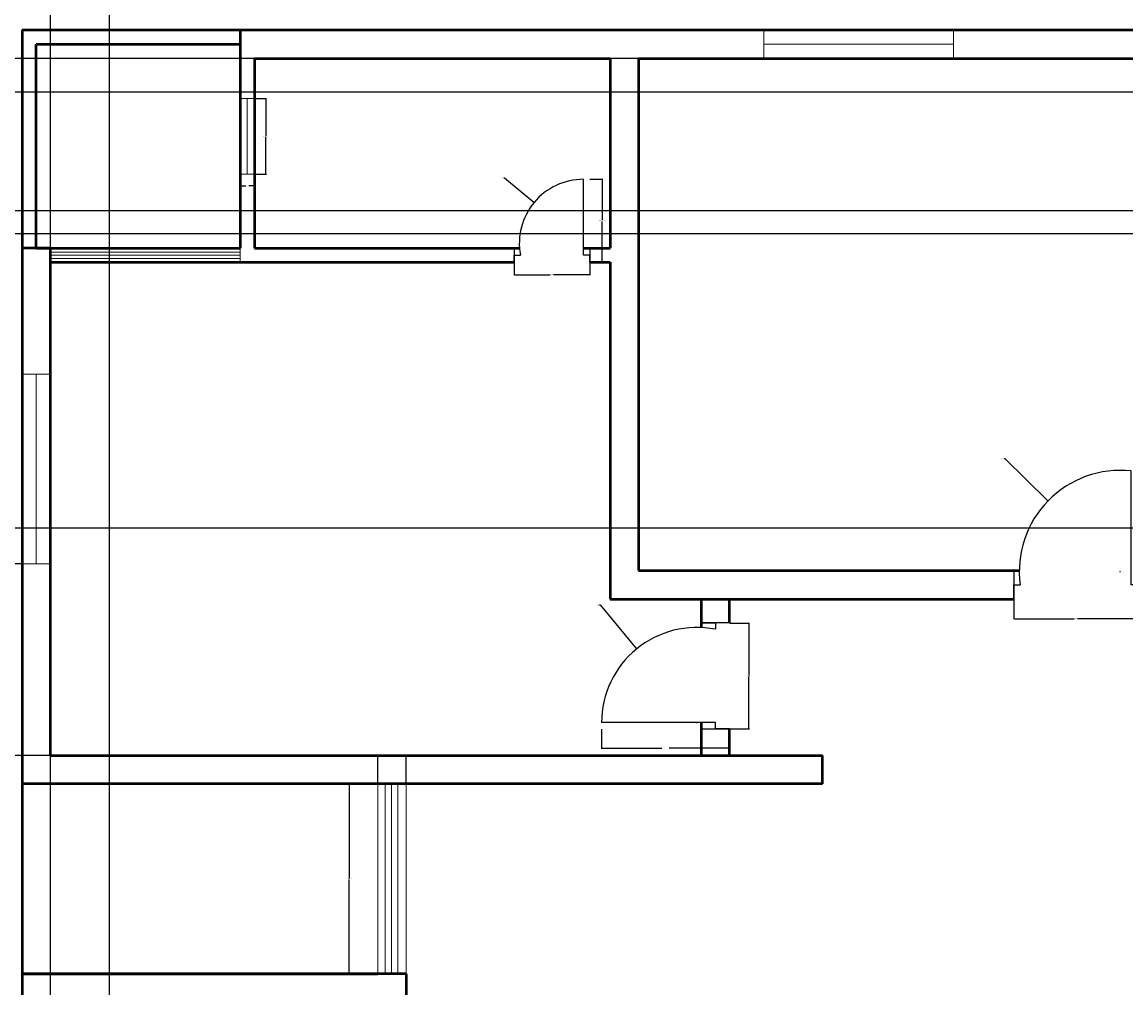
# Model space of a CAD drawing. Units: inches. Extents: x 2215 to 3724, y 1009 to 2124.
# Tile 9 of 11: x 2963 to 3312, y 1444 to 1750. Entities that reach past the tile are written whole.
import ezdxf

# ---------------------------------------------------------------- set-up
doc = ezdxf.new("R2010")
doc.units = ezdxf.units.IN
for name, color, linetype, lineweight in [('A-ANNO-DIMS', 2, 'Continuous', 18), ('A-ANNO-SYMB', 7, 'Continuous', 25), ('A-DOOR', 3, 'Continuous', 25), ('A-GLAZ', 4, 'Continuous', 18), ('A-WALL', 7, 'Continuous', 50)]:
    doc.layers.add(name, color=color, linetype=linetype, lineweight=lineweight)
doc.styles.get("Standard").update_dxf_attribs({"font": 'arial.ttf'})
doc.dimstyles.get("Standard").update_dxf_attribs({"dimtxt": 0.18, "dimasz": 0.18, "dimexe": 0.18, "dimexo": 0.0625, "dimgap": 0.09, "dimtad": 0, "dimtih": 1, "dimtoh": 1, "dimdec": 4, "dimzin": 0, "dimdsep": 46, "dimtxsty": 'Standard', "dimcen": 0.09, "dimadec": 0, "dimazin": 0, "dimtfac": 1, "dimtdec": 4, "dimtofl": 0, "dimtmove": 0, "dimatfit": 3, "dimfxl": 1, "dimtolj": 1, "dimtzin": 0, "dimarcsym": 0})

# ---------------------------------------------------------------- blocks, each defined once
blk = doc.blocks.new('DOOR-BEDROOM-N')
for p, q in [((37.14, 4.5), (37.14, 40.5)), ((0, 9), (0, 0)), ((39.14, 9), (39.14, 0)), ((0, 0), (0, 4.5)), ((0, 4.5), (2, 4.5)), ((39.14, 4.5), (37.14, 4.5)), ((39.14, 0), (39.14, 4.5))]:
    blk.add_line(p, q)
blk.add_arc((33.66, 8.74), 31.95, 83.7441, 187.635)
blk = doc.blocks.new('DOOR-BATH-NW')
for p, q in [((21.95, 2.25), (21.95, 26.25)), ((0, 4.5), (0, 0)), ((23.95, 4.5), (23.95, 0)), ((0, 0), (0, 2.25)), ((0, 2.25), (2, 2.25)), ((23.95, 2.25), (21.95, 2.25)), ((23.95, 0), (23.95, 2.25))]:
    blk.add_line(p, q)
blk.add_arc((21.95, 5.96), 20.29, 90, 190.5328)
blk = doc.blocks.new('DOOR-BEDROOM-W')
for p, q in [((40.5, 33.52), (31.5, 33.52)), ((31.5, 33.52), (36, 33.52)), ((36, 33.52), (36, 31.52)), ((36, 2), (0, 2)), ((31.5, 0), (40.5, 0)), ((36, 0), (36, 2)), ((40.5, 0), (36, 0))]:
    blk.add_line(p, q)
blk.add_arc((30.1, 2), 30.1, 78.701, 180)
blk = doc.blocks.new('WIN-60-JAMB-A')
for p, q in [((0, 9), (0, 0)), ((60, 4.5), (60, 9)), ((60, 9), (60, 0)), ((0, 0), (0, 4.5)), ((0, 4.5), (60, 4.5))]:
    blk.add_line(p, q)
blk = doc.blocks.new('SCREEN-LAUNDRY')
for p, q in [((0, 0), (0, 60)), ((0, 60), (9, 60)), ((4.37, 60), (2.37, 60)), ((2.37, 60), (2.37, 0)), ((4.37, 0), (4.37, 60)), ((6.37, 0), (6.37, 60)), ((9, 60), (9, 0)), ((2.37, 0), (4.37, 0)), ((9, 0), (4.37, 0)), ((4.37, 0), (6.37, 0))]:
    blk.add_line(p, q)
blk = doc.blocks.new('VENT-24-NW')
for p, q in [((0, 24), (0, 24)), ((0, 24), (4.5, 24)), ((4.5, 24), (0, 24)), ((0, 24), (2.25, 24)), ((2.25, 24), (2.25, 0)), ((2.25, 0), (0, 0)), ((0, 0), (0, 0)), ((0, 0), (4.5, 0))]:
    blk.add_line(p, q)
blk = doc.blocks.new('WIN-OTS-W')
for p, q in [((60, 4.5), (60, 0)), ((0, 2.25), (0, 3.25)), ((0, 3.25), (60, 3.25)), ((60, 2.25), (0, 2.25)), ((60, 1.25), (0, 1.25)), ((60, 3.25), (60, 2.25)), ((60, 0), (60, 2.25)), ((60, 2.25), (60, 1.25))]:
    blk.add_line(p, q)
blk = doc.blocks.new('*D39')
at = {"layer": 'A-ANNO-DIMS', "color": 0, "lineweight": -2, "transparency": 16777216}
for p, q in [((3075.18, 1509), (3066.06, 1509)), ((3066.24, 1508.82), (3066.24, 1479.18)), ((3066.24, 1449.18), (3066.24, 1478.81)), ((3075.18, 1449), (3066.06, 1449))]:
    blk.add_line(p, q, dxfattribs=at)
at = {"layer": 'A-ANNO-DIMS', "color": 0, "transparency": 16777216}
for points in [[(3066.21, 1508.82), (3066.27, 1508.82), (3066.24, 1509)], [(3066.21, 1449.18), (3066.27, 1449.18), (3066.24, 1449)]]:
    blk.add_solid(points, dxfattribs=at)
at = {"layer": 'Defpoints', "color": 0, "transparency": 16777216}
for p in [(3066.24, 1509), (3075.24, 1509), (3075.24, 1449)]:
    blk.add_point(p, dxfattribs=at)
at = {"layer": 'A-ANNO-DIMS', "color": 0, "transparency": 16777216, "insert": (3066.24, 1479), "char_height": 0.18, "attachment_point": 5}
blk.add_mtext('\\A1;SCREEN 60 TYP.', dxfattribs=at)
blk = doc.blocks.new('*D40')
at = {"layer": 'A-ANNO-DIMS', "color": 0, "lineweight": -2, "transparency": 16777216}
for p, q in [((3075.24, 1509.06), (3075.24, 1518.18)), ((3075.42, 1518), (3079.29, 1518)), ((3084.06, 1518), (3080.2, 1518)), ((3084.24, 1509.06), (3084.24, 1518.18))]:
    blk.add_line(p, q, dxfattribs=at)
at = {"layer": 'A-ANNO-DIMS', "color": 0, "transparency": 16777216}
for points in [[(3075.42, 1518.03), (3075.42, 1517.97), (3075.24, 1518)], [(3084.06, 1518.03), (3084.06, 1517.97), (3084.24, 1518)]]:
    blk.add_solid(points, dxfattribs=at)
at = {"layer": 'Defpoints', "color": 0, "transparency": 16777216}
for p in [(3084.24, 1518), (3075.24, 1509), (3084.24, 1509)]:
    blk.add_point(p, dxfattribs=at)
at = {"layer": 'A-ANNO-DIMS', "color": 0, "transparency": 16777216, "insert": (3079.74, 1518), "char_height": 0.18, "attachment_point": 5}
blk.add_mtext('\\A1;9 TYP.', dxfattribs=at)
blk = doc.blocks.new('*D41')
at = {"layer": 'A-ANNO-DIMS', "color": 0, "lineweight": -2, "transparency": 16777216}
for p, q in [((3036.31, 1725.83), (3040.02, 1725.83)), ((3039.84, 1725.65), (3039.84, 1714.01)), ((3039.84, 1702.01), (3039.84, 1713.65)), ((3036.31, 1701.83), (3040.02, 1701.83))]:
    blk.add_line(p, q, dxfattribs=at)
at = {"layer": 'A-ANNO-DIMS', "color": 0, "transparency": 16777216}
for points in [[(3039.81, 1725.65), (3039.87, 1725.65), (3039.84, 1725.83)], [(3039.81, 1702.01), (3039.87, 1702.01), (3039.84, 1701.83)]]:
    blk.add_solid(points, dxfattribs=at)
at = {"layer": 'Defpoints', "color": 0, "transparency": 16777216}
for p in [(3036.24, 1725.83), (3039.84, 1725.83), (3036.24, 1701.83)]:
    blk.add_point(p, dxfattribs=at)
at = {"layer": 'A-ANNO-DIMS', "color": 0, "transparency": 16777216, "insert": (3039.84, 1713.83), "char_height": 0.18, "attachment_point": 5}
blk.add_mtext('\\A1;VENT 24 TYP.', dxfattribs=at)
blk = doc.blocks.new('*D42')
at = {"layer": 'A-ANNO-DIMS', "color": 0, "lineweight": -2, "transparency": 16777216}
for p, q in [((3031.74, 1701.77), (3031.74, 1698.05)), ((3036.24, 1701.77), (3036.24, 1698.05)), ((3031.92, 1698.23), (3033.54, 1698.23)), ((3036.06, 1698.23), (3034.45, 1698.23))]:
    blk.add_line(p, q, dxfattribs=at)
at = {"layer": 'A-ANNO-DIMS', "color": 0, "transparency": 16777216}
for points in [[(3031.92, 1698.26), (3031.92, 1698.2), (3031.74, 1698.23)], [(3036.06, 1698.26), (3036.06, 1698.2), (3036.24, 1698.23)]]:
    blk.add_solid(points, dxfattribs=at)
at = {"layer": 'Defpoints', "color": 0, "transparency": 16777216}
for p in [(3031.74, 1701.83), (3036.24, 1701.83), (3036.24, 1698.23)]:
    blk.add_point(p, dxfattribs=at)
at = {"layer": 'A-ANNO-DIMS', "color": 0, "transparency": 16777216, "insert": (3033.99, 1698.23), "char_height": 0.18, "attachment_point": 5}
blk.add_mtext('\\A1;5 TYP.', dxfattribs=at)
blk = doc.blocks.new('*D62')
at = {"layer": 'A-ANNO-DIMS', "color": 0, "lineweight": -2, "transparency": 16777216}
for p, q in [((3276.5, 1567.43), (3276.5, 1561.08)), ((3315.64, 1567.43), (3315.64, 1561.08)), ((3276.68, 1561.26), (3295.54, 1561.26)), ((3315.46, 1561.26), (3296.6, 1561.26))]:
    blk.add_line(p, q, dxfattribs=at)
at = {"layer": 'A-ANNO-DIMS', "color": 0, "transparency": 16777216}
for points in [[(3276.68, 1561.29), (3276.68, 1561.23), (3276.5, 1561.26)], [(3315.46, 1561.29), (3315.46, 1561.23), (3315.64, 1561.26)]]:
    blk.add_solid(points, dxfattribs=at)
at = {"layer": 'Defpoints', "color": 0, "transparency": 16777216}
for p in [(3276.5, 1567.5), (3315.64, 1567.5), (3315.64, 1561.26)]:
    blk.add_point(p, dxfattribs=at)
at = {"layer": 'A-ANNO-DIMS', "color": 0, "transparency": 16777216, "insert": (3296.07, 1561.26), "char_height": 0.18, "attachment_point": 5}
blk.add_mtext('\\A1;39 TYP.', dxfattribs=at)
blk = doc.blocks.new('*D63')
at = {"layer": 'A-ANNO-DIMS', "color": 0, "lineweight": -2, "transparency": 16777216}
for p, q in [((3142.4, 1700.25), (3146.45, 1700.25)), ((3146.27, 1700.07), (3146.27, 1687.31)), ((3146.27, 1674.18), (3146.27, 1686.94)), ((3142.4, 1674), (3146.45, 1674))]:
    blk.add_line(p, q, dxfattribs=at)
at = {"layer": 'A-ANNO-DIMS', "color": 0, "transparency": 16777216}
for points in [[(3146.24, 1700.07), (3146.3, 1700.07), (3146.27, 1700.25)], [(3146.24, 1674.18), (3146.3, 1674.18), (3146.27, 1674)]]:
    blk.add_solid(points, dxfattribs=at)
at = {"layer": 'Defpoints', "color": 0, "transparency": 16777216}
for p in [(3142.33, 1700.25), (3146.27, 1700.25), (3142.33, 1674)]:
    blk.add_point(p, dxfattribs=at)
at = {"layer": 'A-ANNO-DIMS', "color": 0, "transparency": 16777216, "insert": (3146.27, 1687.12), "char_height": 0.18, "attachment_point": 5}
blk.add_mtext('\\A1;WC DOOR 26 TYP.', dxfattribs=at)
blk = doc.blocks.new('*D64')
at = {"layer": 'A-ANNO-DIMS', "color": 0, "lineweight": -2, "transparency": 16777216}
for p, q in [((3118.39, 1673.93), (3118.39, 1669.88)), ((3142.33, 1673.93), (3142.33, 1669.88)), ((3118.57, 1670.06), (3129.83, 1670.06)), ((3142.15, 1670.06), (3130.89, 1670.06))]:
    blk.add_line(p, q, dxfattribs=at)
at = {"layer": 'A-ANNO-DIMS', "color": 0, "transparency": 16777216}
for points in [[(3118.57, 1670.09), (3118.57, 1670.03), (3118.39, 1670.06)], [(3142.15, 1670.09), (3142.15, 1670.03), (3142.33, 1670.06)]]:
    blk.add_solid(points, dxfattribs=at)
at = {"layer": 'Defpoints', "color": 0, "transparency": 16777216}
for p in [(3118.39, 1674), (3142.33, 1674), (3142.33, 1670.06)]:
    blk.add_point(p, dxfattribs=at)
at = {"layer": 'A-ANNO-DIMS', "color": 0, "transparency": 16777216, "insert": (3130.36, 1670.06), "char_height": 0.18, "attachment_point": 5}
blk.add_mtext('\\A1;24 TYP.', dxfattribs=at)
blk = doc.blocks.new('*D65')
at = {"layer": 'A-ANNO-DIMS', "color": 0, "lineweight": -2, "transparency": 16777216}
for p, q in [((3146.06, 1526.33), (3146.06, 1520.14)), ((3186.56, 1526.33), (3186.56, 1520.14)), ((3146.24, 1520.32), (3165.17, 1520.32)), ((3186.38, 1520.32), (3167.46, 1520.32))]:
    blk.add_line(p, q, dxfattribs=at)
at = {"layer": 'A-ANNO-DIMS', "color": 0, "transparency": 16777216}
for points in [[(3146.24, 1520.35), (3146.24, 1520.29), (3146.06, 1520.32)], [(3186.38, 1520.35), (3186.38, 1520.29), (3186.56, 1520.32)]]:
    blk.add_solid(points, dxfattribs=at)
at = {"layer": 'Defpoints', "color": 0, "transparency": 16777216}
for p in [(3146.06, 1526.4), (3186.56, 1526.4), (3186.56, 1520.32)]:
    blk.add_point(p, dxfattribs=at)
at = {"layer": 'A-ANNO-DIMS', "color": 0, "transparency": 16777216, "insert": (3166.31, 1520.32), "char_height": 0.18, "attachment_point": 5}
blk.add_mtext('\\A1;BR DOOR 41 TYP.', dxfattribs=at)
blk = doc.blocks.new('*D66')
at = {"layer": 'A-ANNO-DIMS', "color": 0, "lineweight": -2, "transparency": 16777216}
for p, q in [((3186.63, 1559.91), (3192.82, 1559.91)), ((3192.64, 1559.73), (3192.64, 1543.34)), ((3192.64, 1526.58), (3192.64, 1542.97)), ((3186.63, 1526.4), (3192.82, 1526.4))]:
    blk.add_line(p, q, dxfattribs=at)
at = {"layer": 'A-ANNO-DIMS', "color": 0, "transparency": 16777216}
for points in [[(3192.61, 1559.73), (3192.67, 1559.73), (3192.64, 1559.91)], [(3192.61, 1526.58), (3192.67, 1526.58), (3192.64, 1526.4)]]:
    blk.add_solid(points, dxfattribs=at)
at = {"layer": 'Defpoints', "color": 0, "transparency": 16777216}
for p in [(3186.56, 1559.91), (3192.64, 1559.91), (3186.56, 1526.4)]:
    blk.add_point(p, dxfattribs=at)
at = {"layer": 'A-ANNO-DIMS', "color": 0, "transparency": 16777216, "insert": (3192.64, 1543.15), "char_height": 0.18, "attachment_point": 5}
blk.add_mtext('\\A1;34 TYP.', dxfattribs=at)
blk = doc.blocks.new('*D91')
at = {"layer": 'A-ANNO-DIMS', "color": 0, "lineweight": -2, "transparency": 16777216}
for p, q in [((2962.68, 1578.61), (2877.61, 1578.61)), ((2877.79, 1578.43), (2877.79, 1548.49)), ((2877.79, 1518.18), (2877.79, 1548.12)), ((2971.68, 1518), (2877.61, 1518))]:
    blk.add_line(p, q, dxfattribs=at)
at = {"layer": 'A-ANNO-DIMS', "color": 0, "transparency": 16777216}
for points in [[(2877.76, 1578.43), (2877.82, 1578.43), (2877.79, 1578.61)], [(2877.76, 1518.18), (2877.82, 1518.18), (2877.79, 1518)]]:
    blk.add_solid(points, dxfattribs=at)
at = {"layer": 'Defpoints', "color": 0, "transparency": 16777216}
for p in [(2877.79, 1578.61), (2962.74, 1578.61), (2971.74, 1518)]:
    blk.add_point(p, dxfattribs=at)
at = {"layer": 'A-ANNO-DIMS', "color": 0, "transparency": 16777216, "insert": (2877.79, 1548.3), "char_height": 0.18, "attachment_point": 5}
blk.add_mtext('\\A1;60.61', dxfattribs=at)
blk = doc.blocks.new('*D97')
at = {"layer": 'A-ANNO-DIMS', "color": 0, "lineweight": -2, "transparency": 16777216}
for p, q in [((3520.81, 1747.5), (3590.27, 1747.5)), ((3590.09, 1747.32), (3590.09, 1449.93)), ((3590.09, 1152.18), (3590.09, 1449.57)), ((3259.81, 1152), (3590.27, 1152))]:
    blk.add_line(p, q, dxfattribs=at)
at = {"layer": 'A-ANNO-DIMS', "color": 0, "transparency": 16777216}
for points in [[(3590.06, 1747.32), (3590.12, 1747.32), (3590.09, 1747.5)], [(3590.06, 1152.18), (3590.12, 1152.18), (3590.09, 1152)]]:
    blk.add_solid(points, dxfattribs=at)
at = {"layer": 'Defpoints', "color": 0, "transparency": 16777216}
for p in [(3520.74, 1747.5), (3590.09, 1747.5), (3259.74, 1152)]:
    blk.add_point(p, dxfattribs=at)
at = {"layer": 'A-ANNO-DIMS', "color": 0, "transparency": 16777216, "insert": (3590.09, 1449.75), "char_height": 0.18, "attachment_point": 5}
blk.add_mtext('\\A1;595.5', dxfattribs=at)
blk = doc.blocks.new('*D124')
at = {"layer": 'A-ANNO-DIMS', "color": 0, "lineweight": -2, "transparency": 16777216}
for p, q in [((3334.68, 1690.31), (2877.61, 1690.31)), ((2877.79, 1690.13), (2877.79, 1686.83)), ((2877.79, 1683.18), (2877.79, 1686.47)), ((3334.68, 1683), (2877.61, 1683))]:
    blk.add_line(p, q, dxfattribs=at)
at = {"layer": 'A-ANNO-DIMS', "color": 0, "transparency": 16777216}
for points in [[(2877.76, 1690.13), (2877.82, 1690.13), (2877.79, 1690.31)], [(2877.76, 1683.18), (2877.82, 1683.18), (2877.79, 1683)]]:
    blk.add_solid(points, dxfattribs=at)
at = {"layer": 'Defpoints', "color": 0, "transparency": 16777216}
for p in [(2877.79, 1690.31), (3334.74, 1690.31), (3334.74, 1683)]:
    blk.add_point(p, dxfattribs=at)
at = {"layer": 'A-ANNO-DIMS', "color": 0, "transparency": 16777216, "insert": (2877.79, 1686.65), "char_height": 0.18, "attachment_point": 5}
blk.add_mtext('\\A1;7.31', dxfattribs=at)
blk = doc.blocks.new('*D125')
at = {"layer": 'A-ANNO-DIMS', "color": 0, "lineweight": -2, "transparency": 16777216}
for p, q in [((3405.18, 1738.5), (2877.61, 1738.5)), ((2877.79, 1738.32), (2877.79, 1733.33)), ((2877.79, 1727.97), (2877.79, 1732.96)), ((3405.18, 1727.79), (2877.61, 1727.79))]:
    blk.add_line(p, q, dxfattribs=at)
at = {"layer": 'A-ANNO-DIMS', "color": 0, "transparency": 16777216}
for points in [[(2877.76, 1738.32), (2877.82, 1738.32), (2877.79, 1738.5)], [(2877.76, 1727.97), (2877.82, 1727.97), (2877.79, 1727.79)]]:
    blk.add_solid(points, dxfattribs=at)
at = {"layer": 'Defpoints', "color": 0, "transparency": 16777216}
for p in [(2877.79, 1738.5), (3405.24, 1738.5), (3405.24, 1727.79)]:
    blk.add_point(p, dxfattribs=at)
at = {"layer": 'A-ANNO-DIMS', "color": 0, "transparency": 16777216, "insert": (2877.79, 1733.14), "char_height": 0.18, "attachment_point": 5}
blk.add_mtext('\\A1;10.706', dxfattribs=at)
blk = doc.blocks.new('*D127')
at = {"layer": 'A-ANNO-DIMS', "color": 0, "lineweight": -2, "transparency": 16777216}
for p, q in [((2971.74, 1440.06), (2971.74, 1780.83)), ((2971.92, 1780.65), (2980.62, 1780.65)), ((2990.24, 1780.65), (2981.53, 1780.65)), ((2990.42, 1440.06), (2990.42, 1780.83))]:
    blk.add_line(p, q, dxfattribs=at)
at = {"layer": 'A-ANNO-DIMS', "color": 0, "transparency": 16777216}
for points in [[(2971.92, 1780.68), (2971.92, 1780.62), (2971.74, 1780.65)], [(2990.24, 1780.68), (2990.24, 1780.62), (2990.42, 1780.65)]]:
    blk.add_solid(points, dxfattribs=at)
at = {"layer": 'Defpoints', "color": 0, "transparency": 16777216}
for p in [(2990.42, 1780.65), (2971.74, 1440), (2990.42, 1440)]:
    blk.add_point(p, dxfattribs=at)
at = {"layer": 'A-ANNO-DIMS', "color": 0, "transparency": 16777216, "insert": (2981.08, 1780.65), "char_height": 0.18, "attachment_point": 5}
blk.add_mtext('\\A1;18.673', dxfattribs=at)
blk = doc.blocks.new('*D133')
at = {"layer": 'A-ANNO-DIMS', "color": 0, "lineweight": -2, "transparency": 16777216}
for p, q in [((3273.41, 1611.95), (3273.59, 1611.95)), ((3273.59, 1611.95), (3287.17, 1598.68)), ((3310.07, 1576.24), (3310.25, 1576.24)), ((3310.16, 1576.15), (3310.16, 1576.33))]:
    blk.add_line(p, q, dxfattribs=at)
at = {"layer": 'A-ANNO-DIMS', "color": 0, "transparency": 16777216}
blk.add_solid([(3287.19, 1598.7), (3287.15, 1598.66), (3287.3, 1598.56)], dxfattribs=at)
at = {"layer": 'Defpoints', "color": 0, "transparency": 16777216}
for p in [(3287.3, 1598.56), (3310.16, 1576.24)]:
    blk.add_point(p, dxfattribs=at)
at = {"layer": 'A-ANNO-DIMS', "color": 0, "transparency": 16777216, "insert": (3272.86, 1611.95), "char_height": 0.18, "attachment_point": 5}
blk.add_mtext('\\A1;R31.946', dxfattribs=at)
blk = doc.blocks.new('*D135')
at = {"layer": 'A-ANNO-DIMS', "color": 0, "lineweight": -2, "transparency": 16777216}
for p, q in [((3145.45, 1565.64), (3145.63, 1565.64)), ((3145.63, 1565.64), (3156.97, 1551.81)), ((3176.08, 1528.4), (3176.26, 1528.4)), ((3176.17, 1528.31), (3176.17, 1528.49))]:
    blk.add_line(p, q, dxfattribs=at)
at = {"layer": 'A-ANNO-DIMS', "color": 0, "transparency": 16777216}
blk.add_solid([(3156.99, 1551.83), (3156.94, 1551.79), (3157.08, 1551.67)], dxfattribs=at)
at = {"layer": 'Defpoints', "color": 0, "transparency": 16777216}
for p in [(3157.08, 1551.67), (3176.17, 1528.4)]:
    blk.add_point(p, dxfattribs=at)
at = {"layer": 'A-ANNO-DIMS', "color": 0, "transparency": 16777216, "insert": (3145.06, 1565.64), "char_height": 0.18, "attachment_point": 5}
blk.add_mtext('\\A1;R30.1', dxfattribs=at)
blk = doc.blocks.new('*D141')
at = {"layer": 'A-ANNO-DIMS', "color": 0, "lineweight": -2, "transparency": 16777216}
for p, q in [((3115.19, 1700.71), (3115.37, 1700.71)), ((3115.37, 1700.71), (3124.59, 1693.04)), ((3140.24, 1679.96), (3140.42, 1679.96)), ((3140.33, 1679.87), (3140.33, 1680.05))]:
    blk.add_line(p, q, dxfattribs=at)
at = {"layer": 'A-ANNO-DIMS', "color": 0, "transparency": 16777216}
blk.add_solid([(3124.61, 1693.06), (3124.57, 1693.02), (3124.73, 1692.93)], dxfattribs=at)
at = {"layer": 'Defpoints', "color": 0, "transparency": 16777216}
for p in [(3124.73, 1692.93), (3140.33, 1679.96)]:
    blk.add_point(p, dxfattribs=at)
at = {"layer": 'A-ANNO-DIMS', "color": 0, "transparency": 16777216, "insert": (3114.71, 1700.71), "char_height": 0.18, "attachment_point": 5}
blk.add_mtext('\\A1;R20.29', dxfattribs=at)

msp = doc.modelspace()

# ---------------------------------------------------------------- linework, layer by layer
at = {"layer": 'A-ANNO-SYMB'}
msp.add_line((2910.9414, 1589.9969), (3556.9429, 1589.9969), dxfattribs=at)
at = {"layer": 'A-WALL'}
for p, q in [((2962.7432, 1747.4969), (2962.7432, 1517.9969)), ((2962.7432, 1747.4969), (3520.7432, 1747.4969)), ((3031.7432, 1747.4969), (3031.7432, 1678.4969)), ((2967.2432, 1678.4969), (2967.2432, 1742.9969)), ((2967.2432, 1742.9969), (3031.7432, 1742.9969)), ((3036.2432, 1738.4969), (3036.2432, 1678.4969)), ((3036.2432, 1738.4969), (3148.7432, 1738.4969)), ((3148.7432, 1738.4969), (3148.7432, 1678.4969)), ((3157.7432, 1738.4969), (3157.7432, 1576.4969)), ((3157.7432, 1738.4969), (3325.7432, 1738.4969)), ((3157.7432, 1738.4969), (3157.7432, 1576.4969)), ((2971.7432, 1678.4969), (2962.7432, 1678.4969)), ((2967.2432, 1678.4969), (3031.7432, 1678.4969)), ((2971.7432, 1678.4969), (2967.2432, 1678.4969)), ((2971.7432, 1673.9969), (2971.7432, 1678.4969)), ((3036.2432, 1678.4969), (3120.0959, 1678.4969)), ((3140.3342, 1678.4969), (3148.7432, 1678.4969)), ((2971.7432, 1673.9969), (3118.3852, 1673.9969)), ((2971.7432, 1517.9969), (2971.7432, 1673.9969)), ((3142.3342, 1673.9969), (3148.7432, 1673.9969)), ((3148.7432, 1673.9969), (3148.7432, 1567.4969)), ((3157.7432, 1576.4969), (3278.2152, 1576.4969)), ((3157.7432, 1576.4969), (3278.2152, 1576.4969)), ((3157.7432, 1576.4969), (3278.2152, 1576.4969)), ((3148.7432, 1567.4969), (3276.4974, 1567.4969)), ((3177.5645, 1567.4969), (3177.5645, 1558.4648)), ((3186.5645, 1559.9139), (3186.5645, 1567.4969)), ((3177.5645, 1528.3952), (3177.5645, 1517.9969)), ((3186.5645, 1517.9969), (3186.5645, 1526.3952)), ((2962.7432, 1517.9969), (2962.7432, 1151.9969)), ((2971.7432, 1517.9969), (3215.9113, 1517.9969)), ((3177.5645, 1517.9969), (3177.5645, 1517.9969)), ((3177.5645, 1517.9969), (3186.5645, 1517.9969)), ((3215.9113, 1508.9969), (3215.9113, 1517.9969)), ((3215.9113, 1508.9969), (2962.7432, 1508.9969)), ((3084.2432, 1448.9969), (2962.7432, 1448.9969)), ((2962.7432, 1448.9969), (3075.2432, 1448.9969)), ((3084.2432, 1448.9969), (3084.2432, 1429.4651))]:
    msp.add_line(p, q, dxfattribs=at)

# ---------------------------------------------------------------- block references
at = {"layer": 'A-DOOR'}
for name, p in [('DOOR-BATH-NW', (3118.3852, 1673.997)), ('DOOR-BEDROOM-N', (3276.4972, 1567.497)), ('DOOR-BEDROOM-W', (3146.0642, 1526.395))]:
    msp.add_blockref(name, p, dxfattribs=at)
at = {"layer": 'A-GLAZ'}
for name, p in [('WIN-60-JAMB-A', (3197.3512, 1738.497)), ('VENT-24-NW', (3031.7432, 1701.83)), ('WIN-OTS-W', (2971.7432, 1673.997)), ('SCREEN-LAUNDRY', (3075.2432, 1448.997))]:
    msp.add_blockref(name, p, dxfattribs=at)
at = {"layer": 'A-GLAZ', "rotation": 270.0000000000003}
msp.add_blockref('WIN-60-JAMB-A', (2962.7433, 1638.611), dxfattribs=at)

# ---------------------------------------------------------------- dimensions: what is measured, and where the dimension line sits
at = {"layer": 'A-ANNO-DIMS'}
dim = msp.add_linear_dim(base=(2990.4162, 1780.6469), p1=(2971.7432, 1439.9969), p2=(2990.4162, 1439.9969), dimstyle='Standard', override={"dimdec": 3, "dimlfac": 1, "dimrnd": 0, "dimzin": 0, "dimdsep": 46, "dimlunit": 2}, dxfattribs=at)
dim.commit()
dim.dimension.update_dxf_attribs({"geometry": '*D127', "text_midpoint": (2981.0797, 1780.6469)})
for base, p1, p2, override, picture, middle in [((3590.0929, 1747.4969), (3259.7432, 1151.9969), (3520.7432, 1747.4969), {"dimdec": 1, "dimlfac": 1, "dimrnd": 0, "dimzin": 0, "dimdsep": 46, "dimlunit": 2}, '*D97', (3590.0929, 1449.7469)), ((2877.7914, 1738.4969), (3405.2432, 1727.7909), (3405.2432, 1738.4969), {"dimdec": 3, "dimlfac": 1, "dimrnd": 0, "dimzin": 0, "dimdsep": 46, "dimlunit": 2}, '*D125', (2877.7914, 1733.1439)), ((2877.7914, 1690.3077), (3334.7432, 1682.9969), (3334.7432, 1690.3077), {"dimdec": 2, "dimlfac": 1, "dimrnd": 0, "dimzin": 0, "dimdsep": 46, "dimlunit": 2}, '*D124', (2877.7914, 1686.6523)), ((2877.7914, 1578.6109), (2971.7432, 1517.9969), (2962.7432, 1578.6109), {"dimdec": 2, "dimlfac": 1, "dimrnd": 0, "dimzin": 0, "dimdsep": 46, "dimlunit": 2}, '*D91', (2877.7914, 1548.3039))]:
    dim = msp.add_linear_dim(base=base, p1=p1, p2=p2, angle=90, dimstyle='Standard', override=override, dxfattribs=at)
    dim.commit()
    dim.dimension.update_dxf_attribs({"geometry": picture, "text_midpoint": middle})
for base, p1, p2, text, picture, middle in [((3039.8432, 1725.8303), (3036.2432, 1701.8303), (3036.2432, 1725.8303), 'VENT <> TYP.', '*D41', (3039.8432, 1713.8303)), ((3146.2717, 1700.2469), (3142.3342, 1673.9969), (3142.3342, 1700.2469), 'WC DOOR <> TYP.', '*D63', (3146.2717, 1687.1219)), ((3192.6395, 1559.9139), (3186.5645, 1526.3952), (3186.5645, 1559.9139), '<> TYP.', '*D66', (3192.6395, 1543.1545)), ((3066.2432, 1508.9969), (3075.2432, 1448.9969), (3075.2432, 1508.9969), 'SCREEN <> TYP.', '*D39', (3066.2432, 1478.9969))]:
    dim = msp.add_linear_dim(base=base, p1=p1, p2=p2, angle=90, text=text, dimstyle='Standard', override={"dimdec": 0, "dimlfac": 1, "dimrnd": 0, "dimzin": 0, "dimdsep": 46, "dimlunit": 2}, dxfattribs=at)
    dim.commit()
    dim.dimension.update_dxf_attribs({"geometry": picture, "text_midpoint": middle})
for base, p1, p2, text, picture, middle in [((3036.2432030508, 1698.2302878401), (3031.7432030508, 1701.8302878401), (3036.2432030508, 1701.8302878401), '<> TYP.', '*D42', (3033.9932030508, 1698.2302878401)), ((3142.3342, 1670.0594), (3118.3852, 1673.9969), (3142.3342, 1673.9969), '<> TYP.', '*D64', (3130.3597, 1670.0594)), ((3315.6412, 1561.2614), (3276.4974, 1567.4969), (3315.6412, 1567.4969), '<> TYP.', '*D62', (3296.0693, 1561.2614)), ((3186.5645417523, 1520.3202008817), (3146.0645417523, 1526.3952008817), (3186.5645417523, 1526.3952008817), 'BR DOOR <> TYP.', '*D65', (3166.3145417523, 1520.3202008817)), ((3084.2432, 1517.9969), (3075.2432, 1508.9969), (3084.2432, 1508.9969), '<> TYP.', '*D40', (3079.7432, 1517.9969))]:
    dim = msp.add_linear_dim(base=base, p1=p1, p2=p2, text=text, dimstyle='Standard', override={"dimdec": 0, "dimlfac": 1, "dimrnd": 0, "dimzin": 0, "dimdsep": 46, "dimlunit": 2}, dxfattribs=at)
    dim.commit()
    dim.dimension.update_dxf_attribs({"geometry": picture, "text_midpoint": middle})
for center, mpoint, override, picture, middle in [((3140.3342, 1679.9561), (3124.7298, 1692.9261), {"dimdec": 2, "dimlfac": 1, "dimrnd": 0, "dimzin": 0, "dimdsep": 46, "dimlunit": 2}, '*D141', (3114.7072, 1700.7082)), ((3310.16, 1576.2413), (3287.3009, 1598.5571), {"dimdec": 3, "dimlfac": 1, "dimrnd": 0, "dimzin": 0, "dimdsep": 46, "dimlunit": 2}, '*D133', (3272.8556, 1611.9467)), ((3176.1667, 1528.3952), (3157.0802, 1551.6728), {"dimdec": 1, "dimlfac": 1, "dimrnd": 0, "dimzin": 0, "dimdsep": 46, "dimlunit": 2}, '*D135', (3145.0558, 1565.6393))]:
    dim = msp.add_radius_dim(center=center, mpoint=mpoint, dimstyle='Standard', override=override, dxfattribs=at)
    dim.commit()
    dim.dimension.update_dxf_attribs({"geometry": picture, "text_midpoint": middle, "dimtype": 164})

doc.saveas('drawing.dxf')
